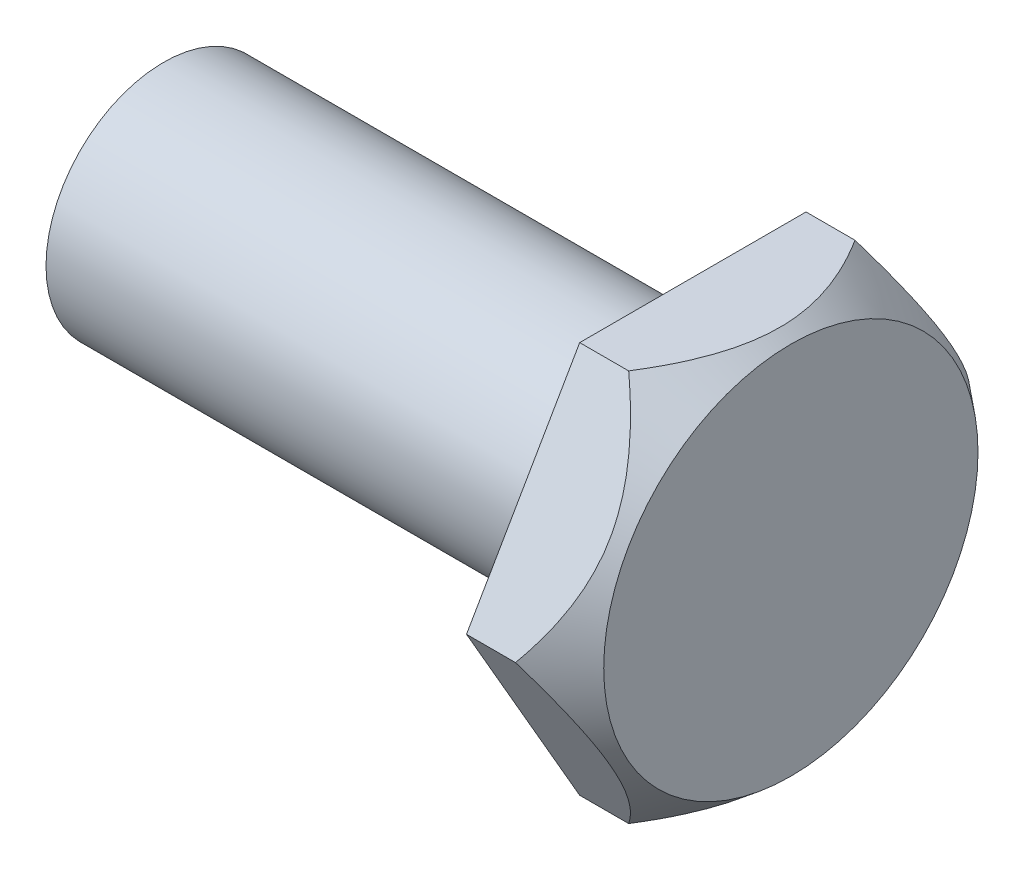
SolidWorks part; units mm, degrees
material "Plain Carbon Steel"
ref_plane "Front Plane" through (0, 0, 0) normal (0, 0, 1) x (1, 0, 0)
ref_plane "Top Plane" through (0, 0, 0) normal (0, 1, 0) x (1, 0, 0)
ref_plane "Right Plane" through (0, 0, 0) normal (1, 0, 0) x (0, 0, -1)
sketch "Hex Head Profile 20AF" plane through (0, 0, 0) normal (1, 0, 0) x (0, 0, -1)
  line L1 (11.547, 0) -> (5.7735, 10)
  line L2 (5.7735, 10) -> (-5.7735, 10)
  line L3 (-5.7735, 10) -> (-11.547, 0)
  line L4 (-11.547, 0) -> (-5.7735, -10)
  line L5 (-5.7735, -10) -> (5.7735, -10)
  line L6 (5.7735, -10) -> (11.547, 0)
  circle A0 centre (0, 0) radius 10 construction
  dimension "D1" = 20
extrude "Hex Head" add sketch "Hex Head Profile 20AF" along normal blind 5
sketch "Shank Profile Ø12" plane through (0, 0, 0) normal (-1, 0, 0) x (0, 0, 1)
  circle A0 centre (0, 0) radius 6
  dimension "D1" = 12
extrude "Shank Ø12" add sketch "Shank Profile Ø12" along normal blind 27
sketch "Head Chamfer Profile" plane through (0, 0, 0) normal (0, 1, 0) x (1, 0, 0)
  line L0 (0, 0) -> (8.6617, 0) construction
  line L1 (2.5, 11.547) -> (5, 9.547)
  line L2 (5, 11.547) -> (0, 11.547) construction
  line L3 (5, 11.547) -> (5, 5.7735) construction
  line L4 (5, 9.547) -> (5, 11.547)
  line L5 (2.5, 11.547) -> (5, 11.547)
  dimension "D1" = 2
revolve "Head Chamfer" cut sketch "Head Chamfer Profile" angle 360 about L0
